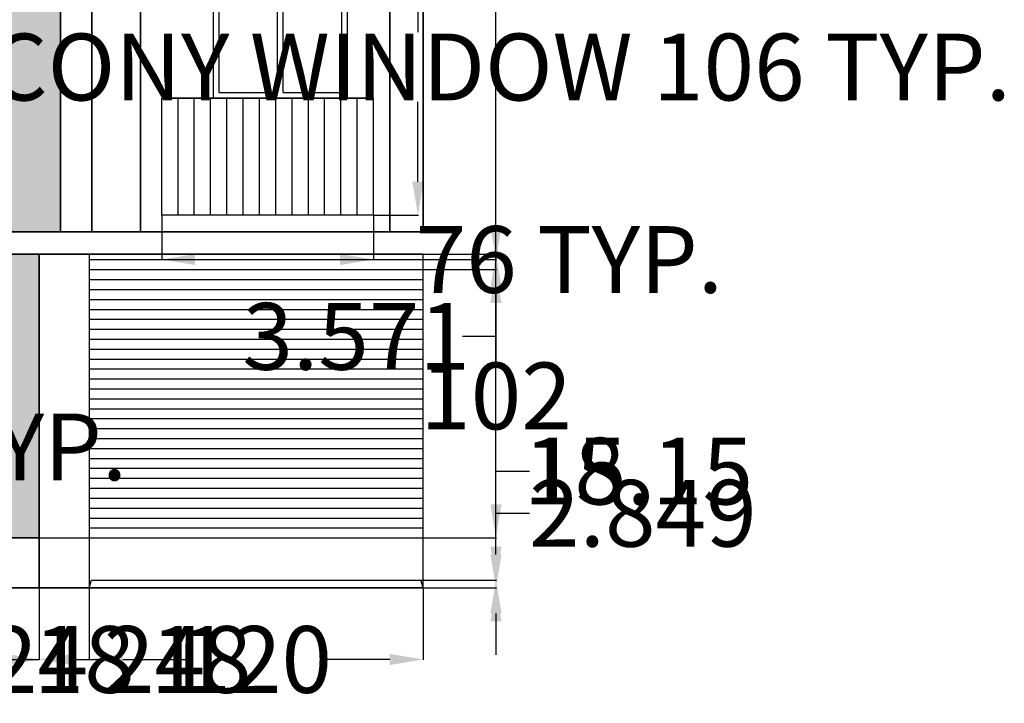
# Model space of a CAD drawing. Units: inches. Extents: x 172 to 828, y 190 to 777.
# Tile 4 of 9: x 474 to 828, y 190 to 436. Entities that reach past the tile are written whole.
import ezdxf

# ---------------------------------------------------------------- set-up
doc = ezdxf.new("R2010")
doc.units = ezdxf.units.IN
doc.header["$MEASUREMENT"] = 0
for name, color, linetype, lineweight in [('A-ANNO-DIMS', 2, 'Continuous', 18), ('A-DOOR', 4, 'Continuous', 25), ('A-ELEV', 7, 'Continuous', 35), ('A-ELEV-PATT', 8, 'Continuous', 13), ('A-GLAZ', 3, 'Continuous', 25)]:
    doc.layers.add(name, color=color, linetype=linetype, lineweight=lineweight)
doc.styles.get("Standard").update_dxf_attribs({"font": 'arial.ttf'})
doc.dimstyles.get("Standard").update_dxf_attribs({"dimtxt": 24, "dimasz": 12, "dimexe": 0.18, "dimexo": 0.0625, "dimgap": 0.09, "dimtad": 0, "dimtih": 1, "dimtoh": 1, "dimdec": 0, "dimzin": 0, "dimdsep": 46, "dimlunit": 3, "dimtxsty": 'Standard', "dimcen": 0.09, "dimadec": 0, "dimazin": 0, "dimtfac": 1, "dimtdec": 0, "dimtofl": 0, "dimtmove": 0, "dimatfit": 3, "dimfxl": 1, "dimtolj": 1, "dimtzin": 0, "dimarcsym": 0})
pattern_1 = [(228.012788, (0.72, 1), (-8, -9), [0.134536, -13.319088]), (184.969741, (0.63, 0.9), (12, 1), [0.230868, -22.8559248]), (132.510447, (0.4, 0.88), (10, -11), [0.162788, -16.1160326]), (267.273689, (0.01, 0.63), (1, 20), [0.210238, -20.813558]), (292.833654, (0, 0.42), (-5, 12), [0.206155, -20.4093731]), (357.273689, (0.08, 0.23), (-20, 1), [0.210238, -20.813558]), (37.6942405, (0.29, 0.22), (-13, -10), [0.278029, -27.5248485]), (72.2553284, (0.51, 0.39), (7, 22), [0.262488, -25.9863215]), (121.4295656, (0.59, 0.64), (-8, 13), [0.21095, -20.8840731]), (175.236358, (0.48, 0.82), (11, -1), [0.240832, -11.8007626]), (222.397438, (0.24, 0.84), (-12, -11), [0.311448, -30.833375]), (138.814075, (1, 0.62), (-7, 6), [0.106301, -10.5238448]), (171.4692344, (0.92, 0.69), (13, -2), [0.202237, -20.0215114]), (225, (0.72, 0.72), (-1e-16, -1), [0.141421, -1.2727926]), (203.19859, (0.65, 0.84), (5, 2), [0.076158, -7.5396151]), (291.80141, (0.58, 0.81), (-1, 3), [0.107703, -5.2774618]), (30.963757, (0.62, 0.71), (3, 2), [0.174929, -5.6560229]), (161.56505, (0.77, 0.8), (2, -1), [0.126491, -3.0357867]), (16.38954, (0, 0.81), (10, 3), [0.1772, -17.5428451]), (70.346176, (0.17, 0.86), (-4, -11), [0.148661, -14.7174077]), (293.19859, (0.77, 1), (-2, 5), [0.152315, -7.4634581]), (343.61046, (0.83, 0.86), (-10, 3), [0.1772, -17.5428451]), (339.443955, (0, 0.19), (-5, 2), [0.17088, -8.3731237]), (294.775141, (0.16, 0.13), (-5, 11), [0.143178, -14.1746431]), (66.80141, (0.78, 0), (2, 5), [0.152315, -7.4634581]), (17.354025, (0.84, 0.14), (-13, -4), [0.167631, -16.5954236]), (69.443955, (0.29, 0), (-2, -5), [0.08544, -8.4585637]), (101.309932, (0.72, 0), (-1, 4), [0.05099, -5.0480295]), (165.963757, (0.71, 0.05), (3, -1), [0.206155, -3.9169506]), (186.009006, (0.51, 0.1), (10, 1), [0.19105, -18.9139232]), (303.690068, (0.62, 0.62), (-1, 2), [0.144222, -3.4613293]), (353.1572266, (0.7, 0.5), (17, -2), [0.251794, -24.9275626]), (60.945396, (0.95, 0.47), (-4, -7), [0.102956, -10.1926741]), (90, (1, 0.56), (-1, 1), [0.06, -0.94]), (120.256437, (0.49, 0.13), (4, -7), [0.138924, -13.75352]), (48.012788, (0.42, 0.25), (8, 9), [0.269072, -13.184552]), (0, (0.6, 0.45), (1, 1), [0.26, -0.74]), (325.3048465, (0.86, 0.45), (10, -7), [0.158114, -15.6532743]), (254.054604, (0.99, 0.36), (-1, -4), [0.145602, -7.1345079]), (207.6459754, (0.95, 0.22), (-19, -10), [0.237065, -23.4694742]), (175.426079, (0.74, 0.11), (-13, 1), [0.250799, -24.8290734])]

# ---------------------------------------------------------------- blocks, each defined once
blk = doc.blocks.new('WIN-BALCONY')
for p, q in [((41.59, 44), (41.59, 104.41)), ((43.59, 44), (43.59, 104.41)), ((76.13, 42), (0, 42)), ((0, 0), (0, 42)), ((5.86, 0), (5.86, 42)), ((11.71, 0), (11.71, 42)), ((17.57, 0), (17.57, 42)), ((23.43, 0), (23.43, 42)), ((29.28, 0), (29.28, 42)), ((35.14, 0), (35.14, 42)), ((40.99, 0), (40.99, 42)), ((46.85, 0), (46.85, 42)), ((52.71, 0), (52.71, 42)), ((58.56, 0), (58.56, 42)), ((64.42, 0), (64.42, 42)), ((70.28, 0), (70.28, 42)), ((76.13, 0), (76.13, 42)), ((76.13, 0), (0, 0))]:
    blk.add_line(p, q)
blk.add_lwpolyline([(18.47, 42), (66.72, 42), (66.72, 106.41), (18.47, 106.41)], close=True)
for points in [[(41.59, 104.41), (20.47, 104.41), (20.47, 44), (41.59, 44)], [(43.59, 44), (64.72, 44), (64.72, 104.41), (43.59, 104.41)]]:
    blk.add_lwpolyline(points)
blk = doc.blocks.new('*D4')
at = {"layer": 'A-ANNO-DIMS', "color": 0, "lineweight": -2, "transparency": 16777216}
for p, q in [((601.02, 471.8), (617.1, 471.8)), ((616.92, 459.8), (616.92, 431.1)), ((616.92, 377.39), (616.92, 406.09)), ((601.02, 365.39), (617.1, 365.39))]:
    blk.add_line(p, q, dxfattribs=at)
at = {"layer": 'A-ANNO-DIMS', "color": 0, "transparency": 16777216}
for points in [[(614.92, 459.8), (618.92, 459.8), (616.92, 471.8)], [(614.92, 377.39), (618.92, 377.39), (616.92, 365.39)]]:
    blk.add_solid(points, dxfattribs=at)
at = {"layer": 'Defpoints', "color": 0, "transparency": 16777216}
for p in [(600.96, 471.8), (616.92, 471.8), (600.96, 365.39)]:
    blk.add_point(p, dxfattribs=at)
at = {"layer": 'A-ANNO-DIMS', "color": 0, "transparency": 16777216, "insert": (616.92, 418.6), "char_height": 24, "attachment_point": 5}
blk.add_mtext('\\A1;BALCONY WINDOW 106 TYP.', dxfattribs=at)
blk = doc.blocks.new('*D5')
at = {"layer": 'A-ANNO-DIMS', "color": 0, "lineweight": -2, "transparency": 16777216}
for p, q in [((524.83, 365.33), (524.83, 349.25)), ((600.96, 365.33), (600.96, 349.25)), ((536.83, 349.43), (588.96, 349.43)), ((600.96, 349.43), (612.96, 349.43))]:
    blk.add_line(p, q, dxfattribs=at)
at = {"layer": 'A-ANNO-DIMS', "color": 0, "transparency": 16777216}
for points in [[(536.83, 351.43), (536.83, 347.43), (524.83, 349.43)], [(588.96, 351.43), (588.96, 347.43), (600.96, 349.43)]]:
    blk.add_solid(points, dxfattribs=at)
at = {"layer": 'Defpoints', "color": 0, "transparency": 16777216}
for p in [(524.83, 365.39), (600.96, 365.39), (600.96, 349.43)]:
    blk.add_point(p, dxfattribs=at)
at = {"layer": 'A-ANNO-DIMS', "color": 0, "transparency": 16777216, "insert": (671.36, 349.43), "char_height": 24, "attachment_point": 5}
blk.add_mtext('\\A1;76 TYP.', dxfattribs=at)
blk = doc.blocks.new('*D8')
at = {"layer": 'A-ANNO-DIMS', "color": 0, "lineweight": -2, "transparency": 16777216}
for p, q in [((340.36, 315.47), (340.36, 327.47)), ((334, 303.47), (340.54, 303.47)), ((334, 260.68), (340.54, 260.68)), ((340.36, 248.68), (340.36, 236.68))]:
    blk.add_line(p, q, dxfattribs=at)
at = {"layer": 'A-ANNO-DIMS', "color": 0, "transparency": 16777216}
for points in [[(338.36, 315.47), (342.36, 315.47), (340.36, 303.47)], [(338.36, 248.68), (342.36, 248.68), (340.36, 260.68)]]:
    blk.add_solid(points, dxfattribs=at)
at = {"layer": 'Defpoints', "color": 0, "transparency": 16777216}
for p in [(333.94, 303.47), (340.36, 303.47), (333.94, 260.68)]:
    blk.add_point(p, dxfattribs=at)
at = {"layer": 'A-ANNO-DIMS', "color": 0, "transparency": 16777216, "insert": (340.36, 282.08), "char_height": 24, "attachment_point": 5}
blk.add_mtext('\\A1;DOOR HANDLE 43 TYP.', dxfattribs=at)
blk = doc.blocks.new('*D10')
at = {"layer": 'A-ANNO-DIMS', "color": 0, "lineweight": -2, "transparency": 16777216}
for p, q in [((258.78, 231.45), (258.78, 761.27)), ((270.78, 761.09), (412.23, 761.09)), ((606.78, 761.09), (465.33, 761.09)), ((618.78, 735.45), (618.78, 761.27))]:
    blk.add_line(p, q, dxfattribs=at)
at = {"layer": 'A-ANNO-DIMS', "color": 0, "transparency": 16777216}
for points in [[(270.78, 763.09), (270.78, 759.09), (258.78, 761.09)], [(606.78, 763.09), (606.78, 759.09), (618.78, 761.09)]]:
    blk.add_solid(points, dxfattribs=at)
at = {"layer": 'Defpoints', "color": 0, "transparency": 16777216}
for p in [(618.78, 761.09), (618.78, 735.39), (258.78, 231.39)]:
    blk.add_point(p, dxfattribs=at)
at = {"layer": 'A-ANNO-DIMS', "color": 0, "transparency": 16777216, "insert": (438.78, 761.09), "char_height": 24, "attachment_point": 5}
blk.add_mtext('\\A1;360', dxfattribs=at)
blk = doc.blocks.new('*D11')
at = {"layer": 'A-ANNO-DIMS', "color": 0, "lineweight": -2, "transparency": 16777216}
for p, q in [((618.84, 735.39), (645.16, 735.39)), ((644.98, 723.39), (644.98, 495.74)), ((644.98, 243.39), (644.98, 471.05)), ((618.84, 231.39), (645.16, 231.39))]:
    blk.add_line(p, q, dxfattribs=at)
at = {"layer": 'A-ANNO-DIMS', "color": 0, "transparency": 16777216}
for points in [[(642.98, 723.39), (646.98, 723.39), (644.98, 735.39)], [(642.98, 243.39), (646.98, 243.39), (644.98, 231.39)]]:
    blk.add_solid(points, dxfattribs=at)
at = {"layer": 'Defpoints', "color": 0, "transparency": 16777216}
for p in [(618.78, 735.39), (644.98, 735.39), (618.78, 231.39)]:
    blk.add_point(p, dxfattribs=at)
at = {"layer": 'A-ANNO-DIMS', "color": 0, "transparency": 16777216, "insert": (644.98, 483.39), "char_height": 24, "attachment_point": 5}
blk.add_mtext('\\A1;504', dxfattribs=at)
blk = doc.blocks.new('*D19')
at = {"layer": 'A-ANNO-DIMS', "color": 0, "lineweight": -2, "transparency": 16777216}
for p, q in [((438.78, 249.33), (438.78, 205.51)), ((414.78, 231.33), (414.78, 205.51)), ((402.78, 205.69), (390.78, 205.69)), ((450.78, 205.69), (462.78, 205.69))]:
    blk.add_line(p, q, dxfattribs=at)
at = {"layer": 'A-ANNO-DIMS', "color": 0, "transparency": 16777216}
for points in [[(402.78, 207.69), (402.78, 203.69), (414.78, 205.69)], [(450.78, 207.69), (450.78, 203.69), (438.78, 205.69)]]:
    blk.add_solid(points, dxfattribs=at)
at = {"layer": 'Defpoints', "color": 0, "transparency": 16777216}
for p in [(438.78, 249.39), (414.78, 231.39), (438.78, 205.69)]:
    blk.add_point(p, dxfattribs=at)
at = {"layer": 'A-ANNO-DIMS', "color": 0, "transparency": 16777216, "insert": (480.21, 205.69), "char_height": 24, "attachment_point": 5}
blk.add_mtext('\\A1;24', dxfattribs=at)
blk = doc.blocks.new('*D20')
at = {"layer": 'A-ANNO-DIMS', "color": 0, "lineweight": -2, "transparency": 16777216}
for p, q in [((438.78, 249.33), (438.78, 205.51)), ((456.78, 249.33), (456.78, 205.51)), ((426.78, 205.69), (414.78, 205.69)), ((468.78, 205.69), (480.78, 205.69))]:
    blk.add_line(p, q, dxfattribs=at)
at = {"layer": 'A-ANNO-DIMS', "color": 0, "transparency": 16777216}
for points in [[(426.78, 207.69), (426.78, 203.69), (438.78, 205.69)], [(468.78, 207.69), (468.78, 203.69), (456.78, 205.69)]]:
    blk.add_solid(points, dxfattribs=at)
at = {"layer": 'Defpoints', "color": 0, "transparency": 16777216}
for p in [(438.78, 249.39), (456.78, 249.39), (456.78, 205.69)]:
    blk.add_point(p, dxfattribs=at)
at = {"layer": 'A-ANNO-DIMS', "color": 0, "transparency": 16777216, "insert": (496.95, 205.69), "char_height": 24, "attachment_point": 5}
blk.add_mtext('\\A1;18', dxfattribs=at)
blk = doc.blocks.new('*D21')
at = {"layer": 'A-ANNO-DIMS', "color": 0, "lineweight": -2, "transparency": 16777216}
for p, q in [((456.78, 249.33), (456.78, 205.51)), ((480.78, 231.33), (480.78, 205.51)), ((444.78, 205.69), (432.78, 205.69)), ((492.78, 205.69), (504.78, 205.69))]:
    blk.add_line(p, q, dxfattribs=at)
at = {"layer": 'A-ANNO-DIMS', "color": 0, "transparency": 16777216}
for points in [[(444.78, 207.69), (444.78, 203.69), (456.78, 205.69)], [(492.78, 207.69), (492.78, 203.69), (480.78, 205.69)]]:
    blk.add_solid(points, dxfattribs=at)
at = {"layer": 'Defpoints', "color": 0, "transparency": 16777216}
for p in [(456.78, 249.39), (480.78, 231.39), (480.78, 205.69)]:
    blk.add_point(p, dxfattribs=at)
at = {"layer": 'A-ANNO-DIMS', "color": 0, "transparency": 16777216, "insert": (522.21, 205.69), "char_height": 24, "attachment_point": 5}
blk.add_mtext('\\A1;24', dxfattribs=at)
blk = doc.blocks.new('*D22')
at = {"layer": 'A-ANNO-DIMS', "color": 0, "lineweight": -2, "transparency": 16777216}
for p, q in [((480.78, 231.33), (480.78, 205.51)), ((498.78, 231.33), (498.78, 205.51)), ((468.78, 205.69), (456.78, 205.69)), ((510.78, 205.69), (522.78, 205.69))]:
    blk.add_line(p, q, dxfattribs=at)
at = {"layer": 'A-ANNO-DIMS', "color": 0, "transparency": 16777216}
for points in [[(468.78, 207.69), (468.78, 203.69), (480.78, 205.69)], [(510.78, 207.69), (510.78, 203.69), (498.78, 205.69)]]:
    blk.add_solid(points, dxfattribs=at)
at = {"layer": 'Defpoints', "color": 0, "transparency": 16777216}
for p in [(480.78, 231.39), (498.78, 231.39), (498.78, 205.69)]:
    blk.add_point(p, dxfattribs=at)
at = {"layer": 'A-ANNO-DIMS', "color": 0, "transparency": 16777216, "insert": (538.95, 205.69), "char_height": 24, "attachment_point": 5}
blk.add_mtext('\\A1;18', dxfattribs=at)
blk = doc.blocks.new('*D23')
at = {"layer": 'A-ANNO-DIMS', "color": 0, "lineweight": -2, "transparency": 16777216}
for p, q in [((498.78, 231.33), (498.78, 205.51)), ((618.78, 231.33), (618.78, 205.51)), ((510.78, 205.69), (533.35, 205.69)), ((606.78, 205.69), (584.21, 205.69))]:
    blk.add_line(p, q, dxfattribs=at)
at = {"layer": 'A-ANNO-DIMS', "color": 0, "transparency": 16777216}
for points in [[(510.78, 207.69), (510.78, 203.69), (498.78, 205.69)], [(606.78, 207.69), (606.78, 203.69), (618.78, 205.69)]]:
    blk.add_solid(points, dxfattribs=at)
at = {"layer": 'Defpoints', "color": 0, "transparency": 16777216}
for p in [(498.78, 231.39), (618.78, 231.39), (618.78, 205.69)]:
    blk.add_point(p, dxfattribs=at)
at = {"layer": 'A-ANNO-DIMS', "color": 0, "transparency": 16777216, "insert": (558.78, 205.69), "char_height": 24, "attachment_point": 5}
blk.add_mtext('\\A1;120', dxfattribs=at)
blk = doc.blocks.new('*D30')
at = {"layer": 'A-ANNO-DIMS', "color": 0, "lineweight": -2, "transparency": 16777216}
for p, q in [((644.98, 261.39), (644.98, 273.39)), ((644.98, 273.39), (656.98, 273.39)), ((480.84, 249.39), (645.16, 249.39)), ((480.84, 231.39), (645.16, 231.39)), ((644.98, 219.39), (644.98, 207.39))]:
    blk.add_line(p, q, dxfattribs=at)
at = {"layer": 'A-ANNO-DIMS', "color": 0, "transparency": 16777216}
for points in [[(642.98, 261.39), (646.98, 261.39), (644.98, 249.39)], [(642.98, 219.39), (646.98, 219.39), (644.98, 231.39)]]:
    blk.add_solid(points, dxfattribs=at)
at = {"layer": 'Defpoints', "color": 0, "transparency": 16777216}
for p in [(480.78, 249.39), (644.98, 249.39), (480.78, 231.39)]:
    blk.add_point(p, dxfattribs=at)
at = {"layer": 'A-ANNO-DIMS', "color": 0, "transparency": 16777216, "insert": (673.15, 273.39), "char_height": 24, "attachment_point": 5}
blk.add_mtext('\\A1;18', dxfattribs=at)
blk = doc.blocks.new('*D31')
at = {"layer": 'A-ANNO-DIMS', "color": 0, "lineweight": -2, "transparency": 16777216}
for p, q in [((480.84, 351.39), (645.16, 351.39)), ((644.98, 339.39), (644.98, 312.74)), ((644.98, 261.39), (644.98, 288.05)), ((480.84, 249.39), (645.16, 249.39))]:
    blk.add_line(p, q, dxfattribs=at)
at = {"layer": 'A-ANNO-DIMS', "color": 0, "transparency": 16777216}
for points in [[(642.98, 339.39), (646.98, 339.39), (644.98, 351.39)], [(642.98, 261.39), (646.98, 261.39), (644.98, 249.39)]]:
    blk.add_solid(points, dxfattribs=at)
at = {"layer": 'Defpoints', "color": 0, "transparency": 16777216}
for p in [(480.78, 351.39), (644.98, 351.39), (480.78, 249.39)]:
    blk.add_point(p, dxfattribs=at)
at = {"layer": 'A-ANNO-DIMS', "color": 0, "transparency": 16777216, "insert": (644.98, 300.39), "char_height": 24, "attachment_point": 5}
blk.add_mtext('\\A1;102', dxfattribs=at)
blk = doc.blocks.new('*D32')
at = {"layer": 'A-ANNO-DIMS', "color": 0, "lineweight": -2, "transparency": 16777216}
for p, q in [((644.98, 246.24), (644.98, 258.24)), ((644.98, 258.24), (656.98, 258.24)), ((618.04, 234.24), (645.16, 234.24)), ((618.84, 231.39), (645.16, 231.39)), ((644.98, 219.39), (644.98, 207.39))]:
    blk.add_line(p, q, dxfattribs=at)
at = {"layer": 'A-ANNO-DIMS', "color": 0, "transparency": 16777216}
for points in [[(642.98, 246.24), (646.98, 246.24), (644.98, 234.24)], [(642.98, 219.39), (646.98, 219.39), (644.98, 231.39)]]:
    blk.add_solid(points, dxfattribs=at)
at = {"layer": 'Defpoints', "color": 0, "transparency": 16777216}
for p in [(617.97, 234.24), (644.98, 234.24), (618.78, 231.39)]:
    blk.add_point(p, dxfattribs=at)
at = {"layer": 'A-ANNO-DIMS', "color": 0, "transparency": 16777216, "insert": (697.79, 258.24), "char_height": 24, "attachment_point": 5}
blk.add_mtext('\\A1;2.849', dxfattribs=at)
blk = doc.blocks.new('*D33')
at = {"layer": 'A-ANNO-DIMS', "color": 0, "lineweight": -2, "transparency": 16777216}
for p, q in [((644.98, 261.39), (644.98, 273.39)), ((644.98, 273.39), (656.98, 273.39)), ((618.84, 249.39), (645.16, 249.39)), ((618.04, 234.24), (645.16, 234.24)), ((644.98, 222.24), (644.98, 210.24))]:
    blk.add_line(p, q, dxfattribs=at)
at = {"layer": 'A-ANNO-DIMS', "color": 0, "transparency": 16777216}
for points in [[(642.98, 261.39), (646.98, 261.39), (644.98, 249.39)], [(642.98, 222.24), (646.98, 222.24), (644.98, 234.24)]]:
    blk.add_solid(points, dxfattribs=at)
at = {"layer": 'Defpoints', "color": 0, "transparency": 16777216}
for p in [(618.78, 249.39), (644.98, 249.39), (617.97, 234.24)]:
    blk.add_point(p, dxfattribs=at)
at = {"layer": 'A-ANNO-DIMS', "color": 0, "transparency": 16777216, "insert": (696.52, 273.39), "char_height": 24, "attachment_point": 5}
blk.add_mtext('\\A1;15.15', dxfattribs=at)
blk = doc.blocks.new('*D34')
at = {"layer": 'A-ANNO-DIMS', "color": 0, "lineweight": -2, "transparency": 16777216}
for p, q in [((618.84, 351.39), (645.16, 351.39)), ((644.98, 339.39), (644.98, 312.74)), ((644.98, 261.39), (644.98, 288.05)), ((618.84, 249.39), (645.16, 249.39))]:
    blk.add_line(p, q, dxfattribs=at)
at = {"layer": 'A-ANNO-DIMS', "color": 0, "transparency": 16777216}
for points in [[(642.98, 339.39), (646.98, 339.39), (644.98, 351.39)], [(642.98, 261.39), (646.98, 261.39), (644.98, 249.39)]]:
    blk.add_solid(points, dxfattribs=at)
at = {"layer": 'Defpoints', "color": 0, "transparency": 16777216}
for p in [(618.78, 351.39), (644.98, 351.39), (618.78, 249.39)]:
    blk.add_point(p, dxfattribs=at)
at = {"layer": 'A-ANNO-DIMS', "color": 0, "transparency": 16777216, "insert": (644.98, 300.39), "char_height": 24, "attachment_point": 5}
blk.add_mtext('\\A1;102', dxfattribs=at)
blk = doc.blocks.new('*D35')
at = {"layer": 'A-ANNO-DIMS', "color": 0, "lineweight": -2, "transparency": 16777216}
for p, q in [((644.98, 361.38), (644.98, 373.38)), ((618.84, 349.38), (645.16, 349.38)), ((618.84, 345.81), (645.16, 345.81)), ((644.98, 333.81), (644.98, 321.81)), ((644.98, 321.81), (632.98, 321.81))]:
    blk.add_line(p, q, dxfattribs=at)
at = {"layer": 'A-ANNO-DIMS', "color": 0, "transparency": 16777216}
for points in [[(642.98, 361.38), (646.98, 361.38), (644.98, 349.38)], [(642.98, 333.81), (646.98, 333.81), (644.98, 345.81)]]:
    blk.add_solid(points, dxfattribs=at)
at = {"layer": 'Defpoints', "color": 0, "transparency": 16777216}
for p in [(618.78, 349.38), (618.78, 345.81), (644.98, 345.81)]:
    blk.add_point(p, dxfattribs=at)
at = {"layer": 'A-ANNO-DIMS', "color": 0, "transparency": 16777216, "insert": (594.72, 321.81), "char_height": 24, "attachment_point": 5}
blk.add_mtext('\\A1;3.571', dxfattribs=at)

msp = doc.modelspace()

# ---------------------------------------------------------------- hatches: boundary and pattern name
at = {"layer": 'A-ELEV-PATT'}
h = msp.add_hatch(dxfattribs=at)
h.set_pattern_fill('GRAVEL', color=256)
h.set_pattern_definition(pattern_1)
h.paths.add_polyline_path([(438.7792, 351.3923), (414.7792, 351.3923), (414.7792, 249.3923), (438.7792, 249.3923)])
h.paths.add_polyline_path([(480.7792, 351.3923), (456.7792, 351.3923), (456.7792, 249.3923), (480.7792, 249.3923)])
h.paths.add_polyline_path([(488.4232, 479.3923), (472.3356, 479.3923), (472.3356, 359.3923), (488.4232, 359.3923)])
h.paths.add_polyline_path([(488.4232, 607.3923), (472.3356, 607.3923), (472.3356, 487.3923), (488.4232, 487.3923)])
h = msp.add_hatch(dxfattribs=at)
h.set_pattern_fill('GRAVEL', color=256)
h.set_pattern_definition(pattern_1)
h.paths.add_polyline_path([(480.7792, 351.3923), (456.7792, 351.3923), (456.7792, 249.3923), (480.7792, 249.3923)])
h.paths.add_polyline_path([(488.4232, 479.3923), (472.3356, 479.3923), (472.3356, 359.3923), (488.4232, 359.3923)])
h.paths.add_polyline_path([(488.4232, 607.3923), (472.3356, 607.3923), (472.3356, 487.3923), (488.4232, 487.3923)])
h = msp.add_hatch(dxfattribs=at)
h.set_pattern_fill('GRAVEL', color=256, scale=20)
h.set_pattern_definition([(228.01279, (14.4, 20), (-160, -180), [2.69072, -266.38176]), (184.96974, (12.6, 18), (240, 20), [4.61736, -457.1185]), (132.51045, (8, 17.6), (200, -220), [3.25576, -322.32065]), (267.27369, (0.2, 12.6), (20, 400), [4.20476, -416.27116]), (292.83365, (0, 8.4), (-100, 240), [4.1231, -408.18746]), (357.27369, (1.6, 4.6), (-400, 20), [4.20476, -416.27116]), (37.69424, (5.8, 4.4), (-260, -200), [5.56058, -550.49697]), (72.25533, (10.2, 7.8), (140, 440), [5.24976, -519.72643]), (121.42957, (11.8, 12.8), (-160, 260), [4.219, -417.68146]), (175.23636, (9.6, 16.4), (220, -20), [4.81664, -236.01525]), (222.39744, (4.8, 16.8), (-240, -220), [6.22896, -616.6675]), (138.81407, (20, 12.4), (-140, 120), [2.126, -210.4769]), (171.46923, (18.4, 13.8), (260, -40), [4.04474, -400.43023]), (225, (14.4, 14.4), (-2e-15, -20), [2.8284, -25.45585]), (203.1986, (13, 16.8), (100, 40), [1.52316, -150.7923]), (291.8014, (11.6, 16.2), (-20, 60), [2.15406, -105.54924]), (30.96376, (12.4, 14.2), (60, 40), [3.4986, -113.12046]), (161.56505, (15.4, 16), (40, -20), [2.5298, -60.71573]), (16.38954, (0, 16.2), (200, 60), [3.544, -350.8569]), (70.34618, (3.4, 17.2), (-80, -220), [2.97322, -294.34815]), (293.1986, (15.4, 20), (-40, 100), [3.0463, -149.26916]), (343.61046, (16.6, 17.2), (-200, 60), [3.544, -350.8569]), (339.44395, (0, 3.8), (-100, 40), [3.4176, -167.46247]), (294.77514, (3.2, 2.6), (-100, 220), [2.86356, -283.49286]), (66.8014, (15.6, 0), (40, 100), [3.0463, -149.26916]), (17.35402, (16.8, 2.8), (-260, -80), [3.35262, -331.90847]), (69.44395, (5.8, 0), (-40, -100), [1.7088, -169.17127]), (101.30993, (14.4, 0), (-20, 80), [1.0198, -100.9606]), (165.96376, (14.2, 1), (60, -20), [4.1231, -78.339]), (186.009, (10.2, 2), (200, 20), [3.821, -378.27846]), (303.6901, (12.4, 12.4), (-20, 40), [2.88444, -69.2266]), (353.15723, (14, 10), (340, -40), [5.03588, -498.55125]), (60.9454, (19, 9.4), (-80, -140), [2.0591, -203.8535]), (90, (20, 11.2), (-20, 20), [1.2, -18.8]), (120.25644, (9.8, 2.6), (80, -140), [2.77848, -275.0704]), (48.01279, (8.4, 5), (160, 180), [5.38144, -263.69104]), (0, (12, 9), (20, 20), [5.2, -14.8]), (325.30485, (17.2, 9), (200, -140), [3.16228, -313.0655]), (254.0546, (19.8, 7.2), (-20, -80), [2.91204, -142.69016]), (207.64598, (19, 4.4), (-380, -200), [4.7413, -469.38948]), (175.42608, (14.8, 2.2), (-260, 20), [5.01598, -496.58147])])
h.paths.add_polyline_path([(480.7792, 351.3923), (456.7792, 351.3923), (456.7792, 249.3923), (480.7792, 249.3923)])
h.paths.add_polyline_path([(472.3356, 479.3923), (464.3356, 479.3923), (464.3356, 359.3923), (472.3356, 359.3923)])
h.paths.add_polyline_path([(488.4232, 479.3923), (472.3356, 479.3923), (472.3356, 359.3923), (488.4232, 359.3923)])
h.paths.add_polyline_path([(472.3356, 607.3923), (464.3356, 607.3923), (464.3356, 487.3923), (472.3356, 487.3923)])
h.paths.add_polyline_path([(488.4232, 607.3923), (472.3356, 607.3923), (472.3356, 487.3923), (488.4232, 487.3923)])

# ---------------------------------------------------------------- linework, layer by layer
at = {"layer": 'A-DOOR'}
for p, q in [((498.7792, 351.3923), (498.7792, 231.3923)), ((618.7792, 231.3923), (618.7792, 351.3923)), ((498.7792, 349.3772), (618.7792, 349.3772)), ((498.7792, 345.8063), (618.7792, 345.8063)), ((498.7792, 342.2354), (618.7792, 342.2354)), ((498.7792, 338.6646), (618.7792, 338.6646)), ((498.7792, 335.0937), (618.7792, 335.0937)), ((498.7792, 331.5228), (618.7792, 331.5228)), ((498.7792, 327.9519), (618.7792, 327.9519)), ((498.7792, 324.381), (618.7792, 324.381)), ((498.7792, 320.8101), (618.7792, 320.8101)), ((498.7792, 317.2392), (618.7792, 317.2392)), ((498.7792, 313.6683), (618.7792, 313.6683)), ((498.7792, 310.0974), (618.7792, 310.0974)), ((498.7792, 306.5265), (618.7792, 306.5265)), ((498.7792, 302.9556), (618.7792, 302.9556)), ((498.7792, 299.3848), (618.7792, 299.3848)), ((498.7792, 295.8139), (618.7792, 295.8139)), ((498.7792, 292.243), (618.7792, 292.243)), ((498.7792, 288.6721), (618.7792, 288.6721)), ((498.7792, 285.1012), (618.7792, 285.1012)), ((498.7792, 281.5303), (618.7792, 281.5303)), ((498.7792, 277.9594), (618.7792, 277.9594)), ((498.7792, 274.3885), (618.7792, 274.3885)), ((498.7792, 270.8176), (618.7792, 270.8176)), ((498.7792, 267.2467), (618.7792, 267.2467)), ((498.7792, 263.6759), (618.7792, 263.6759)), ((498.7792, 260.105), (618.7792, 260.105)), ((498.7792, 256.5341), (618.7792, 256.5341)), ((498.7792, 252.9632), (618.7792, 252.9632)), ((498.7792, 249.3923), (618.7792, 249.3923)), ((498.7792, 231.3923), (499.5849, 234.2412)), ((499.5849, 234.2412), (617.9734, 234.2412)), ((618.7792, 231.3923), (617.9734, 234.2412)), ((498.7792, 231.3923), (618.7792, 231.3923))]:
    msp.add_line(p, q, dxfattribs=at)
at = {"layer": 'A-ELEV'}
for p, q in [((606.8158, 359.3923), (606.8158, 663.3923)), ((618.7792, 359.3923), (618.7792, 663.3923)), ((488.4232, 479.3923), (488.4232, 359.3923)), ((499.6941, 479.3923), (499.6941, 359.3923)), ((517.2267, 479.3923), (517.2267, 359.3923)), ((600.9594, 407.3923), (524.8269, 407.3923)), ((618.7792, 359.3923), (258.7792, 359.3923)), ((618.7792, 351.3923), (258.7792, 351.3923)), ((480.7792, 351.3923), (480.7792, 231.3923)), ((456.7792, 249.3923), (480.7792, 249.3923)), ((258.7792, 231.3923), (618.7792, 231.3923))]:
    msp.add_line(p, q, dxfattribs=at)

# ---------------------------------------------------------------- block references
at = {"layer": 'A-GLAZ'}
msp.add_blockref('WIN-BALCONY', (524.827, 365.392), dxfattribs=at)

# ---------------------------------------------------------------- dimensions: what is measured, and where the dimension line sits
at = {"layer": 'A-ANNO-DIMS'}
for base, p1, p2, picture, middle in [((618.7792, 761.0923), (258.7792, 231.3923), (618.7792, 735.3923), '*D10', (438.7792, 761.0923)), ((438.7792, 205.6923), (414.7792, 231.3923), (438.7792, 249.3923), '*D19', (480.2143, 205.6923)), ((456.7792, 205.6923), (438.7792, 249.3923), (456.7792, 249.3923), '*D20', (496.9538, 205.6923)), ((480.7792, 205.6923), (456.7792, 249.3923), (480.7792, 231.3923), '*D21', (522.2143, 205.6923)), ((498.7792, 205.6923), (480.7792, 231.3923), (498.7792, 231.3923), '*D22', (538.9538, 205.6923)), ((618.7792, 205.6923), (498.7792, 231.3923), (618.7792, 231.3923), '*D23', (558.7792, 205.6923))]:
    dim = msp.add_linear_dim(base=base, p1=p1, p2=p2, dimstyle='Standard', override={"dimdec": 0, "dimlfac": 1, "dimrnd": 0, "dimzin": 0, "dimdsep": 46, "dimlunit": 2}, dxfattribs=at)
    dim.commit()
    dim.dimension.update_dxf_attribs({"geometry": picture, "text_midpoint": middle})
for base, p1, p2, override, picture, middle in [((644.9792, 735.3923), (618.7792, 231.3923), (618.7792, 735.3923), {"dimdec": 0, "dimlfac": 1, "dimrnd": 0, "dimzin": 0, "dimdsep": 46, "dimlunit": 2}, '*D11', (644.9792, 483.3923)), ((644.9792, 345.8063), (618.7792, 349.3772), (618.7792, 345.8063), {"dimdec": 3, "dimlfac": 1, "dimrnd": 0, "dimzin": 0, "dimdsep": 46, "dimlunit": 2}, '*D35', (594.72, 321.8063)), ((644.9792, 351.3923), (480.7792, 249.3923), (480.7792, 351.3923), {"dimdec": 0, "dimlfac": 1, "dimrnd": 0, "dimzin": 0, "dimdsep": 46, "dimlunit": 2}, '*D31', (644.9792, 300.3923)), ((644.9792, 351.3923), (618.7792, 249.3923), (618.7792, 351.3923), {"dimdec": 0, "dimlfac": 1, "dimrnd": 0, "dimzin": 0, "dimdsep": 46, "dimlunit": 2}, '*D34', (644.9792, 300.3923)), ((644.9792, 249.3923), (480.7792, 231.3923), (480.7792, 249.3923), {"dimdec": 0, "dimlfac": 1, "dimrnd": 0, "dimzin": 0, "dimdsep": 46, "dimlunit": 2}, '*D30', (673.1538, 273.3923)), ((644.9792, 249.3923), (617.9734, 234.2412), (618.7792, 249.3923), {"dimdec": 2, "dimlfac": 1, "dimrnd": 0, "dimzin": 0, "dimdsep": 46, "dimlunit": 2}, '*D33', (696.5235, 273.3923)), ((644.9792, 234.2412), (618.7792, 231.3923), (617.9734, 234.2412), {"dimdec": 3, "dimlfac": 1, "dimrnd": 0, "dimzin": 0, "dimdsep": 46, "dimlunit": 2}, '*D32', (697.7922, 258.2412))]:
    dim = msp.add_linear_dim(base=base, p1=p1, p2=p2, angle=90, dimstyle='Standard', override=override, dxfattribs=at)
    dim.commit()
    dim.dimension.update_dxf_attribs({"geometry": picture, "text_midpoint": middle})
for base, p1, p2, text, picture, middle in [((616.9208, 471.8013), (600.9594, 365.3923), (600.9594, 471.8013), 'BALCONY WINDOW <> TYP.', '*D4', (616.9208, 418.5968)), ((340.3606, 303.4742), (333.9412, 260.6781), (333.9412, 303.4742), 'DOOR HANDLE <> TYP.', '*D8', (340.3606, 282.0761))]:
    dim = msp.add_linear_dim(base=base, p1=p1, p2=p2, angle=90, text=text, dimstyle='Standard', override={"dimdec": 0, "dimlfac": 1, "dimrnd": 0, "dimzin": 0, "dimdsep": 46, "dimlunit": 2}, dxfattribs=at)
    dim.commit()
    dim.dimension.update_dxf_attribs({"geometry": picture, "text_midpoint": middle})
dim = msp.add_linear_dim(base=(600.9594, 349.4309), p1=(524.8269, 365.3923), p2=(600.9594, 365.3923), text='<> TYP.', dimstyle='Standard', override={"dimdec": 0, "dimlfac": 1, "dimrnd": 0, "dimzin": 0, "dimdsep": 46, "dimlunit": 2}, dxfattribs=at)
dim.commit()
dim.dimension.update_dxf_attribs({"geometry": '*D5', "text_midpoint": (671.3632, 349.4309)})

doc.saveas('drawing.dxf')
